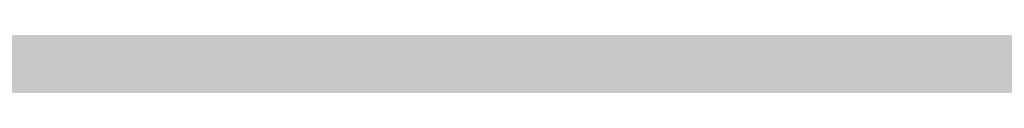
# Model space of a CAD drawing. Units: inches. Extents: x 2091 to 2899, y 967 to 2217.
# Tile 200 of 256: x 2203.18039 to 2203.25707, y 1152.25042 to 1152.25378. Entities that reach past the tile are written whole.
import ezdxf

# ---------------------------------------------------------------- set-up
doc = ezdxf.new("R2010")
doc.units = ezdxf.units.IN
doc.layers.add('A-WALL-PATT', color=141, linetype='Continuous', lineweight=13, true_color=0xadddf7)

msp = doc.modelspace()

# ---------------------------------------------------------------- hatches: boundary and pattern name
at = {"layer": 'A-WALL-PATT'}
h = msp.add_hatch(color=256, dxfattribs=at)
h.dxf.hatch_style = 1
h.paths.add_polyline_path([(2803.143603, 2050.919059), (2203.143603, 2050.919059), (2203.143603, 1090.919059), (2803.143603, 1090.919059)])
h.paths.add_polyline_path([(2635.79885, 1147.540465), (2674.524052, 1147.540465, 0.376086), (2678.529665, 1152.880202), (2678.529665, 1159.556473, 0.333335), (2674.524319, 1163.561846), (2674.524319, 1163.56185), (2674.524319, 1192.93439), (2635.805971, 1192.93439), (2597.087622, 1192.93439), (2597.087622, 1163.561846, 0.333335), (2593.082276, 1159.556473), (2593.082276, 1152.880202, 0.376086), (2597.087889, 1147.540465)], flags=0)
h.paths.add_polyline_path([(2436.010433, 1278.240778, 0.000483), (2435.952643, 1278.215027, -0.001328), (2435.935625, 1278.111693, -0.001711), (2436.11644, 1278.040758, 0.002185)], flags=0)
h.paths.add_polyline_path([(2794.143603, 1143.419059), (2794.143603, 1347.419059), (2543.370171, 1347.419059), (2543.370171, 1351.919059), (2794.143603, 1351.919059), (2794.143603, 1392.713555), (2793.947398, 1392.713555), (2793.947398, 1473.5369), (2794.143603, 1473.5369), (2794.143603, 1531.919059), (2650.143603, 1531.919059), (2650.143603, 1536.419059), (2794.143603, 1536.419059), (2794.143603, 1692.419059), (2609.375609, 1692.419059), (2609.375609, 1644.419059), (2604.875609, 1644.419059), (2604.875609, 1744.919059), (2609.375609, 1744.919059), (2609.375609, 1696.919059), (2794.143603, 1696.919059), (2794.143603, 1780.919059), (2609.643603, 1780.919059), (2493.875609, 1780.919059), (2493.875609, 1785.419059), (2609.643603, 1785.419059), (2794.143603, 1785.419059), (2794.143603, 1847.938821), (2793.951222, 1847.938821), (2793.951222, 1928.762166), (2794.143603, 1928.762166), (2794.143603, 1941.419059), (2614.143603, 1941.419059), (2614.143603, 1821.419059), (2609.643603, 1821.419059), (2609.643603, 1941.419059), (2392.143603, 1941.419059), (2392.143603, 1819.919059), (2387.643603, 1819.919059), (2387.643603, 1941.419059), (2212.143603, 1941.419059), (2212.143603, 1783.919059), (2392.143603, 1783.919059), (2392.143603, 1780.919059), (2212.143603, 1780.919059), (2212.143603, 1629.419059), (2387.643603, 1629.419059), (2387.643603, 1744.919059), (2392.143603, 1744.919059), (2392.143603, 1627.919059), (2317.143603, 1627.919059), (2317.143603, 1551.419059), (2317.143603, 1536.419059), (2459.383591, 1536.419059), (2459.383591, 1602.39648), (2463.883591, 1602.39648), (2463.883591, 1531.919059), (2456.643603, 1531.919059), (2456.643603, 1529.919059), (2452.143603, 1529.919059), (2452.143603, 1531.919059), (2312.643603, 1531.919059), (2312.643603, 1551.419059), (2306.143603, 1551.419059), (2306.143603, 1555.919059), (2308.143603, 1555.919059), (2308.143603, 1551.419059), (2312.643603, 1551.419059), (2312.643603, 1627.919059), (2212.143603, 1627.919059), (2212.143603, 1555.919059), (2270.143603, 1555.919059), (2270.143603, 1551.419059), (2212.143603, 1551.419059), (2212.143603, 1351.919059), (2272.143603, 1351.919059), (2272.143603, 1347.419059), (2212.143603, 1347.419059), (2212.143603, 1275.419059), (2308.143603, 1275.419059), (2308.143603, 1351.919059), (2452.143603, 1351.919059), (2452.143603, 1493.919059), (2456.643603, 1493.919059), (2456.643603, 1347.419059), (2312.643603, 1347.419059), (2312.643603, 1270.919059), (2212.143603, 1270.919059), (2212.143603, 1099.919059), (2281.237523, 1099.919059), (2282.871041, 1110.913803), (2282.008341, 1116.996603), (2278.557741, 1121.420403), (2268.205641, 1128.056203), (2272.087641, 1128.056203), (2273.812941, 1131.927003), (2279.420341, 1134.691903), (2285.027841, 1135.244903), (2287.615841, 1137.456803), (2288.047141, 1138.009803), (2289.341141, 1140.774703), (2291.066541, 1139.668703), (2292.360541, 1135.244903), (2295.379841, 1136.903803), (2296.242541, 1135.797903), (2297.105241, 1133.033003), (2300.124641, 1138.009803), (2303.143941, 1138.009803), (2304.437941, 1135.797903), (2303.143941, 1133.586003), (2306.594641, 1134.691903), (2307.888741, 1133.033003), (2310.908041, 1135.244903), (2313.927441, 1134.138903), (2315.62686, 1132.427102), (2308.320041, 1117.549603), (2290.203841, 1109.807903), (2288.909841, 1103.172103), (2289.272309, 1099.919059), (2434.918227, 1099.919059), (2431.593227, 1124.788059), (2429.930227, 1169.553059), (2430.927185, 1240.519694), (2435.658926, 1238.186126), (2437.135227, 1196.554059), (2438.798227, 1143.973059), (2442.678227, 1111.998059), (2446.558227, 1099.919059), (2794.143603, 1099.919059), (2794.143603, 1138.919059), (2548.032447, 1138.919059), (2548.032447, 1143.419059), (2548.032447, 1148.819059), (2546.668457, 1148.031559), (2528.685692, 1179.178622, 0.256256), (2512.032447, 1148.819059), (2512.032447, 1143.419059), (2512.032447, 1138.919059), (2507.532447, 1138.919059), (2507.532447, 1143.419059), (2507.532447, 1148.819059, 0.256256), (2490.879202, 1179.178622), (2472.896437, 1148.031559), (2471.532447, 1148.819059), (2471.532447, 1143.419059), (2467.032447, 1143.419059), (2467.032447, 1269.945786, 0.039061), (2460.909987, 1273.580059), (2467.032447, 1273.580059), (2467.032447, 1286.325364, 0.014511), (2465.216194, 1286.761905), (2467.032447, 1287.052576), (2467.032447, 1323.419059), (2471.532447, 1323.419059), (2471.532447, 1148.819059), (2489.532447, 1179.995973), (2490.896437, 1179.208473), (2490.879202, 1179.178622, -0.256256), (2507.532447, 1148.819059), (2507.532447, 1143.419059), (2512.032447, 1143.419059), (2512.032447, 1148.819059, -0.256256), (2528.685692, 1179.178622), (2528.668457, 1179.208473), (2530.032447, 1179.995973), (2548.032447, 1148.819059), (2548.032447, 1143.419059)], flags=16)
h.paths.add_polyline_path([(2607.768546, 1200.945083), (2607.768546, 1265.030625), (2597.087622, 1281.052011), (2619.784585, 1281.052011), (2627.795278, 1337.12686), (2635.79885, 1337.12686), (2643.816663, 1337.12686), (2651.827356, 1281.052011), (2674.524319, 1281.052011), (2663.843395, 1265.030625), (2663.843395, 1200.945083), (2635.805971, 1200.945083)], flags=0)
edge = h.paths.add_edge_path(flags=0)
edge.add_ellipse((13303.896215, 1272.998725), major_axis=(-10595.31304, 0.000001), ratio=0.842303870086, start_angle=0.6282372191, end_angle=0.6465540999, ccw=False)
edge.add_ellipse((2711.70045, 1156.852678), major_axis=(2.219769, 0), ratio=0.84230387, start_angle=111.535244, end_angle=180.628237, ccw=False)
edge.add_ellipse((13303.156292, 1272.998725), major_axis=(-10593.026306, 0), ratio=0.842303869544, start_angle=0.5282714718, end_angle=0.6465540971, ccw=False)
edge.add_line((2710.764596, 1175.333295), (2710.129986, 1175.333295))
edge.add_ellipse((2710.129986, 1176.579775), major_axis=(1.479846, 0), ratio=0.84230387, start_angle=180, end_angle=270, ccw=False)
edge.add_line((2708.65014, 1176.579775), (2708.65014, 1200.782914))
edge.add_ellipse((2710.129986, 1200.782914), major_axis=(1.479846, 0), ratio=0.84230387, start_angle=90, end_angle=180, ccw=False)
edge.add_line((2710.129986, 1202.029394), (2710.465075, 1202.029394))
edge.add_ellipse((13303.156292, 1272.998725), major_axis=(-10593.026306, 0), ratio=0.842303869544, start_angle=-0.0902290886, end_angle=0.3838667788, ccw=False)
edge.add_ellipse((2710.129986, 1290.927031), major_axis=(-1.479846, 0), ratio=0.84230387, start_angle=0, end_angle=90, ccw=False)
edge.add_line((2708.65014, 1290.927031), (2708.65014, 1315.13017))
edge.add_ellipse((2710.129986, 1315.13017), major_axis=(-1.479846, 0), ratio=0.84230387, start_angle=-90, end_angle=0, ccw=False)
edge.add_line((2710.129986, 1316.37665), (2710.706314, 1316.37665))
edge.add_ellipse((3238.40172, 1296.289566), major_axis=(528.234, 0), ratio=0.8423038695, start_angle=176.34957241, end_angle=177.82004969, ccw=False)
edge.add_ellipse((2775.063043, 1071.450696), major_axis=(313.307761, 0), ratio=0.8423038695, start_angle=102.12596555, end_angle=103.78052899, ccw=False)
edge.add_ellipse((2775.063043, 1078.305698), major_axis=(-305.302891, 0), ratio=0.8423038695, start_angle=-79.790461, end_angle=-77.55537271, ccw=False)
edge.add_ellipse((2695.141767, 1541.975383), major_axis=(-250.960216, 0), ratio=0.8423038695, start_angle=99.25656601, end_angle=102.55493264)
edge.add_line((2741.410326, 1334.214255), (2747.132545, 1337.378477))
edge.add_ellipse((2747.538616, 1336.857478), major_axis=(-0.739923, 0), ratio=0.8423039, start_angle=270, end_angle=307.93313, ccw=False)
edge.add_ellipse((2747.538616, 1336.857478), major_axis=(-0.739923, 0), ratio=0.8423039, start_angle=232.06687, end_angle=270, ccw=False)
edge.add_line((2747.944687, 1337.378477), (2753.666906, 1334.214255))
edge.add_ellipse((2799.935466, 1541.975383), major_axis=(250.960216, 0), ratio=0.8423038695, start_angle=257.44506736, end_angle=260.74343399)
edge.add_ellipse((2720.014189, 1078.305698), major_axis=(305.302891, 0), ratio=0.8423038695, start_angle=77.55537271, end_angle=79.790461, ccw=False)
edge.add_ellipse((2720.014189, 1071.450696), major_axis=(-313.307761, 0), ratio=0.8423038695, start_angle=256.21947101, end_angle=257.87403445, ccw=False)
edge.add_ellipse((2256.675512, 1296.289566), major_axis=(-528.234, 0), ratio=0.8423038695, start_angle=182.17995031, end_angle=183.65042759, ccw=False)
edge.add_line((2784.370918, 1316.37665), (2784.947247, 1316.37665))
edge.add_ellipse((2784.947247, 1315.13017), major_axis=(1.479846, 0), ratio=0.84230387, start_angle=0, end_angle=90, ccw=False)
edge.add_line((2786.427093, 1315.13017), (2786.427093, 1290.927031))
edge.add_ellipse((2784.947247, 1290.927031), major_axis=(1.479846, 0), ratio=0.84230387, start_angle=270, end_angle=360, ccw=False)
edge.add_ellipse((-7808.07906, 1272.998725), major_axis=(10593.026306, 0), ratio=0.842303869544, start_angle=-0.3838667788, end_angle=0.0902290886, ccw=False)
edge.add_line((2784.612157, 1202.029394), (2784.947247, 1202.029394))
edge.add_ellipse((2784.947247, 1200.782914), major_axis=(1.479846, 0), ratio=0.84230387, start_angle=0, end_angle=90, ccw=False)
edge.add_line((2786.427093, 1200.782914), (2786.427093, 1176.579775))
edge.add_ellipse((2784.947247, 1176.579775), major_axis=(-1.479846, 0), ratio=0.84230387, start_angle=90, end_angle=180, ccw=False)
edge.add_line((2784.947247, 1175.333295), (2784.312636, 1175.333295))
edge.add_ellipse((-7808.07906, 1272.998725), major_axis=(10593.026306, 0), ratio=0.842303869544, start_angle=-0.6186431963, end_angle=-0.5282714718, ccw=False)
edge.add_ellipse((2783.376783, 1156.852678), major_axis=(-2.219769, 0), ratio=0.84230387, start_angle=179.371763, end_angle=248.464757, ccw=False)
edge.add_ellipse((-7808.818983, 1272.998725), major_axis=(-10595.31304, 0.000004), ratio=0.842303865762, start_angle=179.3534459226, end_angle=179.3717628034, ccw=False)
edge.add_ellipse((2780.297303, 1153.500793), major_axis=(-5.246426, 0), ratio=0.84230387, start_angle=90, end_angle=179.353446, ccw=False)
edge.add_line((2780.297303, 1149.081708), (2714.77993, 1149.081708))
edge.add_ellipse((2714.77993, 1153.500793), major_axis=(5.246426, 0), ratio=0.84230387, start_angle=180.646554, end_angle=270, ccw=False)
edge = h.paths.add_edge_path(flags=0)
edge.add_line((2718.187367, 1151.007833), (2718.187367, 1170.472364))
edge.add_ellipse((2721.14706, 1170.472364), major_axis=(-2.959692, 0), ratio=0.84230387, start_angle=-90, end_angle=0, ccw=False)
edge.add_line((2721.14706, 1172.965324), (2773.930173, 1172.965324))
edge.add_ellipse((2773.930173, 1170.472364), major_axis=(-2.959692, 0), ratio=0.84230387, start_angle=180, end_angle=270, ccw=False)
edge.add_line((2776.889865, 1170.472364), (2776.889865, 1151.007833))
edge.add_line((2776.889865, 1151.007833), (2718.187367, 1151.007833))
edge = h.paths.add_edge_path(flags=0)
edge.add_line((2718.187367, 1180.23415), (2718.187367, 1199.057834))
edge.add_ellipse((2747.538616, 1320.39864), major_axis=(147.017924, 0), ratio=0.8423038695, start_angle=256.40186531, end_angle=283.59813469)
edge.add_line((2776.889865, 1199.057834), (2776.889865, 1180.23415))
edge.add_ellipse((2747.538616, 1301.574956), major_axis=(147.017924, 0), ratio=0.8423038695, start_angle=256.40186531, end_angle=283.59813469, ccw=False)
edge = h.paths.add_edge_path(flags=0)
edge.add_ellipse((13303.156292, 1272.998725), major_axis=(-10591.54646, 0), ratio=0.842303869555, start_angle=0.0555943135, end_angle=0.3777641939, ccw=False)
edge.add_line((2711.616859, 1262.72171), (2715.667408, 1249.495396))
edge.add_ellipse((6413.891963, 1241.691919), major_axis=(-3698.236159, 0), ratio=0.84230386955, start_angle=-0.120897369, end_angle=0.364076349)
edge.add_line((2715.761038, 1218.192455), (2711.934307, 1203.167361))
edge = h.paths.add_edge_path(flags=0)
edge.add_line((2718.187367, 1251.074566), (2716.002485, 1267.450435))
edge.add_ellipse((2742.151175, 1202.18954), major_axis=(81.772585, 0), ratio=0.84230387, start_angle=94.27742096, end_angle=111.8349538, ccw=False)
edge.add_line((2737.009748, 1270.930626), (2758.067484, 1270.930626))
edge.add_ellipse((2752.926058, 1202.18954), major_axis=(81.772585, 0), ratio=0.84230387, start_angle=68.1650462, end_angle=85.72257904, ccw=False)
edge.add_line((2779.074747, 1267.450435), (2776.889865, 1251.074566))
edge.add_ellipse((2750.338059, 1187.885356), major_axis=(79.579664, 0), ratio=0.84230387, start_angle=67.20808512, end_angle=85.1299304)
edge.add_line((2756.034656, 1254.743656), (2739.042576, 1254.743656))
edge.add_ellipse((2744.739174, 1187.885356), major_axis=(79.579664, 0), ratio=0.84230387, start_angle=94.8700696, end_angle=112.79191488)
edge = h.paths.add_edge_path(flags=0)
edge.add_line((2783.142926, 1203.167361), (2779.316194, 1218.192455))
edge.add_ellipse((-918.81473, 1241.691919), major_axis=(3698.236159, 0), ratio=0.84230386955, start_angle=-0.364076349, end_angle=0.120897369)
edge.add_line((2779.409825, 1249.495396), (2783.460373, 1262.72171))
edge.add_ellipse((-7808.07906, 1272.998725), major_axis=(-10591.54646, 0), ratio=0.84230386954, start_angle=179.6222358061, end_angle=179.9444056865, ccw=False)
edge = h.paths.add_edge_path(flags=0)
edge.add_ellipse((2734.200892, 1286.69044), major_axis=(-0.356609, 6.340078), ratio=0.60383358, start_angle=89.0020143, end_angle=253.657408, ccw=False)
edge.add_line((2730.369001, 1286.541806), (2730.369001, 1301.35198))
edge.add_line((2730.369001, 1301.35198), (2735.913311, 1305.214803))
edge.add_ellipse((2736.384917, 1304.734561), major_axis=(0.739923, 0), ratio=0.8423039, start_angle=90, end_angle=134.480211, ccw=False)
edge.add_line((2736.384917, 1305.357801), (2738.032783, 1305.357801))
edge.add_line((2738.032783, 1305.357801), (2738.032783, 1307.707927))
edge.add_ellipse((2794.201642, 1307.707927), major_axis=(56.168859, 0), ratio=0.84230387, start_angle=150.5614304, end_angle=180, ccw=False)
edge.add_ellipse((2700.875591, 1307.707927), major_axis=(-56.168859, 0), ratio=0.84230387, start_angle=180, end_angle=209.4385696, ccw=False)
edge.add_line((2757.04445, 1307.707927), (2757.04445, 1305.357801))
edge.add_line((2757.04445, 1305.357801), (2758.692316, 1305.357801))
edge.add_ellipse((2758.692316, 1304.734561), major_axis=(-0.739923, 0), ratio=0.8423039, start_angle=225.519789, end_angle=270, ccw=False)
edge.add_line((2759.163922, 1305.214803), (2764.708231, 1301.35198))
edge.add_line((2764.708231, 1301.35198), (2764.708231, 1286.541806))
edge.add_ellipse((2760.87634, 1286.69044), major_axis=(0.356609, 6.340078), ratio=0.60383358, start_angle=106.342592, end_angle=270.9979857, ccw=False)
edge.add_line((2757.04445, 1285.79709), (2757.04445, 1307.707927))
edge.add_ellipse((2700.875591, 1307.707927), major_axis=(-56.168859, 0), ratio=0.84230387, start_angle=180, end_angle=209.4385696)
edge.add_ellipse((2794.201642, 1307.707927), major_axis=(56.168859, 0), ratio=0.84230387, start_angle=150.5614304, end_angle=180)
edge.add_line((2738.032783, 1307.707927), (2738.032783, 1285.79709))
h.paths.add_polyline_path([(2417.812273, 1104.449704), (2413.492273, 1102.529704), (2410.612273, 1103.969704), (2409.172273, 1106.369704), (2407.252273, 1107.329704), (2406.292273, 1109.729704), (2405.332273, 1114.049704), (2405.332273, 1117.889704), (2406.292273, 1120.129704), (2407.252273, 1119.809704), (2408.848322, 1118.327658), (2410.173945, 1119.42417), (2410.211273, 1120.405704), (2411.040731, 1121.419054), (2410.699273, 1119.858704), (2410.173945, 1119.42417), (2410.088452, 1117.176109), (2411.132836, 1116.206324), (2413.972273, 1119.329704), (2416.852273, 1120.769704), (2416.869721, 1120.798784), (2417.035071, 1119.405116), (2417.896213, 1118.143384), (2418.292273, 1118.369704), (2419.544447, 1120.039269), (2419.360915, 1118.387487), (2419.032108, 1119.356151), (2418.398939, 1118.511926), (2419.252273, 1114.529704), (2418.794091, 1107.198795)], flags=0)
h.paths.add_polyline_path([(2508.870171, 1347.419059), (2508.370171, 1347.419059), (2508.370171, 1351.919059), (2508.870171, 1351.919059)], flags=0)
h.paths.add_polyline_path([(2473.370171, 1347.419059), (2472.370171, 1347.419059), (2467.870171, 1347.419059), (2467.870171, 1455.419059), (2472.370171, 1455.419059), (2472.370171, 1352.419059), (2473.370171, 1352.419059)], flags=0)
h.paths.add_polyline_path([(2352.106244, 1217.446197), (2349.226244, 1218.886197), (2347.786244, 1221.286197), (2345.866244, 1222.246197), (2344.906244, 1224.646197), (2343.946244, 1228.966197), (2343.946244, 1232.806197), (2344.906244, 1235.046197), (2345.866244, 1234.726197), (2347.462293, 1233.244152), (2348.787916, 1234.340663), (2348.825244, 1235.322197), (2349.654702, 1236.335547), (2349.313244, 1234.775197), (2348.787916, 1234.340663), (2348.702423, 1232.092603), (2349.746807, 1231.122817), (2352.586244, 1234.246197), (2355.466244, 1235.686197), (2355.483692, 1235.715277), (2355.649043, 1234.321609), (2356.510185, 1233.059877), (2356.906244, 1233.286197), (2358.158418, 1234.955762), (2357.974887, 1233.30398), (2357.646079, 1234.272644), (2357.012911, 1233.428419), (2357.866244, 1229.446197), (2357.408062, 1222.115288), (2356.426244, 1219.366197)], flags=0)
h.paths.add_polyline_path([(2348.2968, 1112.22442), (2347.0138, 1112.31042), (2345.5298, 1114.12742), (2345.7318, 1115.85842), (2346.8118, 1116.98242), (2346.8118, 1114.64642), (2345.8668, 1114.21442), (2346.8798, 1114.30042)], flags=0)
h.paths.add_polyline_path([(2347.0138, 1110.92642), (2346.2718, 1110.49342), (2346.6098, 1111.18642)], flags=0)
h.paths.add_polyline_path([(2345.8668, 1118.19442), (2345.5298, 1117.32942), (2343.7078, 1118.02142), (2344.3828, 1118.62642)], flags=0)
h.paths.add_polyline_path([(2346.6768, 1109.28242), (2346.0698, 1108.07142), (2345.8668, 1110.06142)], flags=0)
h.paths.add_polyline_path([(2345.0568, 1119.75142), (2343.6398, 1119.75142), (2343.9778, 1121.13542)], flags=0)
h.paths.add_polyline_path([(2345.2598, 1116.55042), (2345.1248, 1115.85842), (2344.9218, 1115.68542), (2344.7198, 1116.37742)], flags=0)
h.paths.add_polyline_path([(2345.6648, 1112.31042), (2345.4618, 1111.53242), (2344.0448, 1111.96442), (2344.6518, 1112.57042)], flags=0)
h.paths.add_polyline_path([(2345.1918, 1113.34942), (2344.4498, 1113.86842), (2344.7198, 1114.38742)], flags=0)
h.paths.add_polyline_path([(2344.6518, 1116.80942), (2344.1798, 1115.68542), (2344.6518, 1115.33942), (2343.9098, 1114.90642), (2343.0328, 1115.94442), (2343.6398, 1116.46342)], flags=0)
h.paths.add_polyline_path([(2345.8668, 1106.68642), (2344.9898, 1105.56242), (2344.5168, 1106.60042)], flags=0)
h.paths.add_polyline_path([(2344.8548, 1110.06142), (2344.5168, 1109.28242), (2344.1128, 1109.71542)], flags=0)
h.paths.add_polyline_path([(2344.0448, 1113.52242), (2343.4378, 1113.08942), (2342.7628, 1113.95442)], flags=0)
h.paths.add_polyline_path([(2344.3148, 1111.01242), (2342.9648, 1110.32042), (2342.9648, 1111.09942)], flags=0)
h.paths.add_polyline_path([(2345.1248, 1104.69742), (2344.5848, 1103.74542), (2344.4498, 1104.26442)], flags=0)
h.paths.add_polyline_path([(2342.8298, 1121.22242), (2341.7498, 1120.53042), (2340.5358, 1121.04942), (2340.1308, 1121.82842), (2340.6708, 1122.95242), (2341.1428, 1121.82842), (2341.6148, 1122.00142)], flags=0)
h.paths.add_polyline_path([(2342.9648, 1119.75142), (2343.0328, 1118.45342), (2342.0878, 1118.02142), (2342.0198, 1119.49142)], flags=0)
h.paths.add_polyline_path([(2342.6948, 1116.89642), (2341.9528, 1116.63642), (2342.0198, 1117.32942)], flags=0)
h.paths.add_polyline_path([(2343.0328, 1112.22442), (2342.0198, 1111.79142), (2341.5478, 1112.22442), (2342.3578, 1113.34942)], flags=0)
h.paths.add_polyline_path([(2343.7748, 1104.43742), (2342.6278, 1102.88042), (2342.6948, 1104.61042), (2343.4378, 1105.12942)], flags=0)
h.paths.add_polyline_path([(2342.0198, 1115.07942), (2340.8058, 1115.51242), (2340.9408, 1116.37742)], flags=0)
h.paths.add_polyline_path([(2341.4808, 1120.09742), (2341.4808, 1119.40542), (2341.0758, 1119.57842), (2341.1428, 1120.09742)], flags=0)
h.paths.add_polyline_path([(2341.8178, 1114.47342), (2340.9408, 1113.08942), (2340.8058, 1114.56042)], flags=0)
h.paths.add_polyline_path([(2341.1428, 1118.54042), (2340.9408, 1116.98242), (2339.0508, 1117.67542), (2339.0508, 1118.62642)], flags=0)
h.paths.add_polyline_path([(2342.6948, 1101.66842), (2341.9528, 1101.84142), (2342.5598, 1102.36142)], flags=0)
h.paths.add_polyline_path([(2340.3328, 1119.66542), (2338.4438, 1119.57842), (2337.9038, 1120.35742), (2339.6578, 1120.61642)], flags=0)
h.paths.add_polyline_path([(2340.3328, 1115.33942), (2340.0628, 1113.69542), (2339.3878, 1115.33942)], flags=0)
h.paths.add_polyline_path([(2341.8178, 1103.83142), (2341.5478, 1102.88042), (2341.1428, 1103.65842)], flags=0)
h.paths.add_polyline_path([(2339.0508, 1122.86642), (2337.2958, 1121.82842), (2337.0938, 1123.12542), (2337.7688, 1123.81842)], flags=0)
h.paths.add_polyline_path([(2339.1178, 1121.74142), (2338.8478, 1121.22242), (2338.1738, 1121.04942), (2338.3758, 1121.56842)], flags=0)
h.paths.add_polyline_path([(2339.1858, 1119.31942), (2338.6458, 1118.71342), (2338.2408, 1118.10742), (2338.2408, 1118.88642)], flags=0)
h.paths.add_polyline_path([(2341.1428, 1101.92842), (2340.6028, 1101.23642), (2340.0628, 1101.84142), (2340.6028, 1102.36142)], flags=0)
h.paths.add_polyline_path([(2337.6338, 1117.76142), (2336.6208, 1118.28042), (2337.2958, 1118.97242)], flags=0)
h.paths.add_polyline_path([(2336.8238, 1119.57842), (2334.7988, 1118.97242), (2335.2038, 1120.35742), (2336.5538, 1120.87642)], flags=0)
h.paths.add_polyline_path([(2339.1178, 1100.45742), (2337.3638, 1100.54342), (2336.7558, 1101.23642)], flags=0)
h.paths.add_polyline_path([(2336.3508, 1122.43342), (2336.0138, 1121.91442), (2334.9338, 1122.43342), (2334.5288, 1123.47142), (2335.7438, 1122.77942)], flags=0)
h.paths.add_polyline_path([(2334.7318, 1120.87642), (2334.2588, 1120.35742), (2334.0568, 1120.78942), (2334.5968, 1121.30842)], flags=0)
h.paths.add_polyline_path([(2334.4618, 1122.17442), (2332.5718, 1121.30842), (2331.3568, 1122.17442), (2332.0998, 1122.86642)], flags=0)
h.paths.add_polyline_path([(2334.2588, 1118.54042), (2333.3818, 1118.45342), (2333.6518, 1119.31942)], flags=0)
h.paths.add_polyline_path([(2335.5418, 1102.27442), (2334.1918, 1102.62042), (2335.2718, 1103.31242)], flags=0)
h.paths.add_polyline_path([(2332.7068, 1119.66542), (2331.6948, 1120.44342), (2332.5048, 1120.78942)], flags=0)
h.paths.add_polyline_path([(2334.7318, 1101.14942), (2333.5168, 1101.58242), (2333.9888, 1101.75542)], flags=0)
h.paths.add_polyline_path([(2332.6398, 1116.63642), (2331.0868, 1116.29042), (2331.9648, 1118.19442)], flags=0)
h.paths.add_polyline_path([(2330.7498, 1121.56842), (2330.2768, 1120.27042), (2328.5228, 1119.31942), (2328.9948, 1121.04942)], flags=0)
h.paths.add_polyline_path([(2330.7498, 1118.62642), (2330.0078, 1117.50242), (2329.8728, 1118.02142)], flags=0)
h.paths.add_polyline_path([(2332.0998, 1102.36142), (2330.5468, 1102.01442), (2331.6948, 1102.96642)], flags=0)
h.paths.add_polyline_path([(2329.5348, 1113.60842), (2329.0628, 1112.31042), (2328.5898, 1113.34942)], flags=0)
h.paths.add_polyline_path([(2328.3878, 1117.84842), (2327.5098, 1116.55042), (2327.1728, 1117.76142)], flags=0)
h.paths.add_polyline_path([(2329.7378, 1106.51342), (2329.5348, 1105.30242), (2328.2528, 1106.08142)], flags=0)
h.paths.add_polyline_path([(2328.6578, 1114.38742), (2328.0498, 1114.12742), (2328.3198, 1114.90642)], flags=0)
h.paths.add_polyline_path([(2328.3198, 1112.22442), (2327.1058, 1112.13742), (2326.7008, 1112.65642)], flags=0)
h.paths.add_polyline_path([(2326.9028, 1115.25242), (2326.7008, 1114.12742), (2325.2158, 1113.60842), (2326.0928, 1115.33942)], flags=0)
h.paths.add_polyline_path([(2326.6328, 1108.33042), (2326.0928, 1107.37942), (2325.8908, 1108.50342), (2326.4978, 1109.10942)], flags=0)
h.paths.add_polyline_path([(2615.143603, 1531.919059), (2609.643603, 1531.919059), (2609.643603, 1620.419059), (2614.143603, 1620.419059), (2614.143603, 1536.419059), (2615.143603, 1536.419059)], flags=0)
h.paths.add_polyline_path([(2545.143603, 1563.419059), (2464.143603, 1563.419059), (2464.143603, 1632.419059), (2509.143603, 1632.419059), (2509.143603, 1627.919059), (2509.143603, 1603.919059), (2468.643603, 1603.919059), (2468.643603, 1567.919059), (2540.643603, 1567.919059), (2540.643603, 1591.919059), (2545.143603, 1591.919059)], flags=0)
h.paths.add_polyline_path([(2388.969048, 1549.985735), (2357.434181, 1549.985735), (2357.434181, 1623.360778), (2399.362777, 1623.360778), (2435.689465, 1623.360778), (2435.592547, 1602.559273), (2435.592547, 1602.39648), (2388.969048, 1602.39648)], flags=0)
h.paths.add_polyline_path([(2388.880628, 1555.809151), (2374.904429, 1555.809151), (2374.904429, 1600.571564), (2374.904429, 1615.457645), (2406.350877, 1615.457645), (2406.350877, 1618.939431), (2412.174293, 1615.457645), (2406.350877, 1611.97586), (2406.350877, 1615.457645), (2388.880628, 1615.457645)], flags=0)
h.paths.add_polyline_path([(2568.875609, 1644.419059), (2453.375609, 1644.419059), (2453.375609, 1785.419059), (2457.875609, 1785.419059), (2457.875609, 1648.919059), (2568.875609, 1648.919059)], flags=0)
h.paths.add_polyline_path([(2212.143603, 1945.919059), (2212.143603, 2041.919059), (2794.143603, 2041.919059), (2794.143603, 1945.919059)], flags=16)
h.paths.add_polyline_path([(2271.082728, 1964.317238), (2776.852968, 1964.317238), (2776.852968, 2037.169623), (2271.082728, 2037.169623)], flags=8)
h.paths.add_polyline_path([(2380.649285, 1536.824144), (2461.040809, 1536.824144), (2461.040809, 1554.652587), (2380.649285, 1554.652587)], flags=8)
h.paths.add_polyline_path([(2240.755709, 1609.725451), (2309.185829, 1609.725451), (2309.185829, 1617.698204), (2240.755709, 1617.698204)], flags=8)
h.paths.add_polyline_path([(2212.677255, 1313.504102), (2282.59152, 1313.504102), (2282.59152, 1322.745239), (2212.677255, 1322.745239)], flags=8)
h.paths.add_polyline_path([(2457.111976, 1114.778574), (2558.481581, 1114.778574), (2558.481581, 1142.219682), (2457.111976, 1142.219682)], flags=8)
h.paths.add_polyline_path([(2473.442337, 1273.010067), (2604.641226, 1273.010067), (2604.641226, 1318.346935), (2473.442337, 1318.346935)], flags=8)
h.paths.add_polyline_path([(2638.876302, 1626.977432), (2684.250367, 1627.976738), (2684.038483, 1637.597494), (2638.664417, 1636.598188)], flags=8)
h.paths.add_polyline_path([(2537.590554, 1453.793447), (2628.389547, 1453.793447), (2628.389547, 1475.344811), (2537.590554, 1475.344811)], flags=8)
h.paths.add_polyline_path([(2504.137638, 1714.632397), (2554.647187, 1714.632397), (2554.647187, 1730.237712), (2504.137638, 1730.237712)], flags=8)
h.paths.add_polyline_path([(2487.501181, 1575.651872), (2535.097121, 1575.651872), (2535.097121, 1598.377646), (2487.501181, 1598.377646)], flags=8)
h.paths.add_polyline_path([(2709.0994, 1735.710278), (2740.016601, 1735.710278), (2740.016601, 1749.937641), (2709.0994, 1749.937641)], flags=8)
h.paths.add_polyline_path([(2442.438424, 1792.171657), (2564.728835, 1792.171657), (2564.728835, 1842.000163), (2442.438424, 1842.000163)], flags=8)
h.paths.add_polyline_path([(2655.815801, 1809.644076), (2789.520142, 1806.693796), (2790.084977, 1832.291638), (2656.380635, 1835.241918)], flags=8)
h.paths.add_polyline_path([(2234.842697, 1797.720143), (2368.592851, 1794.768852), (2369.160718, 1820.504132), (2235.410564, 1823.455423)], flags=8)
h.paths.add_polyline_path([(2245.138466, 1644.006335), (2398.427733, 1640.6239), (2398.994842, 1666.32482), (2245.705575, 1669.707255)], flags=8)
h.paths.add_polyline_path([(2306.142847, 1431.168519), (2413.768314, 1428.793687), (2414.333148, 1454.391529), (2306.707682, 1456.76636)], flags=8)
h.paths.add_polyline_path([(2306.834582, 1458.233145), (2393.380484, 1456.323449), (2393.932808, 1481.354358), (2307.386907, 1483.264054)], flags=8)

doc.saveas('drawing.dxf')
